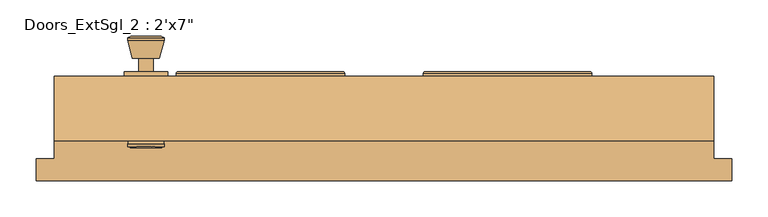
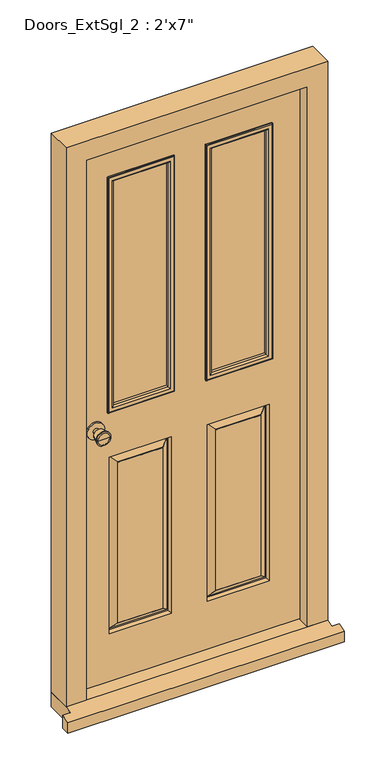
"""IFC4 building model written with IfcOpenShell, lengths in millimetres: door geometry."""

from ifc_helpers import new_model, si_unit, point, frame, frame_2d, origin, place, context, project, spatial, polyline, circle_curve, ellipse_curve, trimmed, segment, composite_curve, outline, extrude, faceted_brep, source, transform, mapped, element, save
from ifc_brep_helpers import plane_surface, cylinder_surface, revolved_surface, advanced_brep


def door_51b0c682(model_context):
    return source(origin(), model_context, "Body", "SolidModel", [
        advanced_brep(
        [(-328.5, 18.4, 1000.0), (-338.5, 18.4, 1000.0), (-318.5, 18.4, 1000.0), (-308.0241324, 67.4, 1000.0), (-348.9758676, 67.4, 1000.0), (-328.5, 67.4, 1000.0), (-303.5, 65.5721319, 1000.0), (-353.5, 65.5721319, 1000.0), (-303.5, 62.1084537, 1000.0), (-353.5, 62.1084537, 1000.0), (-309.863764, 37.4, 1000.0), (-347.136236, 37.4, 1000.0), (-318.5, 37.4, 1000.0), (-338.5, 37.4, 1000.0)],
        [
            (0, 1),
            (1, 2, circle_curve(frame((-328.5, 18.4, 1000.0), z_axis=(0.0, -1.0, 0.0), x_axis=(-1.0, 0.0, 0.0)), 10.0)),
            (2, 0),
            (2, 1, circle_curve(frame((-328.5, 18.4, 1000.0), z_axis=(0.0, -1.0, 0.0), x_axis=(-1.0, 0.0, 0.0)), 10.0)),
            (3, 4, circle_curve(frame((-328.5, 67.4, 1000.0), z_axis=(0.0, 1.0, 0.0), x_axis=(-1.0, 0.0, 0.0)), 20.4758676)),
            (4, 5),
            (5, 3),
            (4, 3, circle_curve(frame((-328.5, 67.4, 1000.0), z_axis=(0.0, 1.0, 0.0), x_axis=(-1.0, 0.0, 0.0)), 20.4758676)),
            (6, 7, circle_curve(frame((-328.5, 65.5721319, 1000.0), z_axis=(0.0, 1.0, 0.0), x_axis=(-1.0, 0.0, 0.0)), 25.0)),
            (7, 4),
            (3, 6),
            (7, 6, circle_curve(frame((-328.5, 65.5721319, 1000.0), z_axis=(0.0, 1.0, 0.0), x_axis=(-1.0, 0.0, 0.0)), 25.0)),
            (8, 9, circle_curve(frame((-328.5, 62.1084537, 1000.0), z_axis=(0.0, 1.0, 0.0), x_axis=(-1.0, 0.0, 0.0)), 25.0)),
            (9, 7),
            (6, 8),
            (9, 8, circle_curve(frame((-328.5, 62.1084537, 1000.0), z_axis=(0.0, 1.0, 0.0), x_axis=(-1.0, 0.0, 0.0)), 25.0)),
            (10, 11, circle_curve(frame((-328.5, 37.4, 1000.0), z_axis=(0.0, 1.0, 0.0), x_axis=(-1.0, 0.0, 0.0)), 18.636236)),
            (11, 9),
            (8, 10),
            (11, 10, circle_curve(frame((-328.5, 37.4, 1000.0), z_axis=(0.0, 1.0, 0.0), x_axis=(-1.0, 0.0, 0.0)), 18.636236)),
            (12, 13, circle_curve(frame((-328.5, 37.4, 1000.0), z_axis=(0.0, 1.0, 0.0), x_axis=(-1.0, 0.0, 0.0)), 10.0)),
            (13, 11),
            (10, 12),
            (13, 12, circle_curve(frame((-328.5, 37.4, 1000.0), z_axis=(0.0, 1.0, 0.0), x_axis=(-1.0, 0.0, 0.0)), 10.0)),
            (1, 13),
            (12, 2),
        ],
        [
            plane_surface(frame((-328.5, 18.4, 1000.0), z_axis=(0.0, -1.0, 0.0), x_axis=(-1.0, 0.0, 0.0))),
            plane_surface(frame((-328.5, 67.4, 1000.0), z_axis=(0.0, 1.0, 0.0), x_axis=(-1.0, 0.0, 0.0))),
            revolved_surface(polyline([(-348.9758676, 67.4, 1000.0), (-353.5, 65.5721319, 1000.0)]), (-328.5, 18.4, 1000.0), (0.0, -1.0, 0.0)),
            cylinder_surface(frame((-328.5, 18.4, 1000.0), z_axis=(0.0, -1.0, 0.0), x_axis=(-1.0, 0.0, 0.0)), 25.0),
            revolved_surface(polyline([(-353.5, 62.1084537, 1000.0), (-347.136236, 37.4, 1000.0)]), (-328.5, 18.4, 1000.0), (0.0, -1.0, 0.0)),
            plane_surface(frame((-328.5, 37.4, 1000.0), z_axis=(0.0, -1.0, 0.0), x_axis=(-1.0, 0.0, 0.0))),
            cylinder_surface(frame((-328.5, 18.4, 1000.0), z_axis=(0.0, -1.0, 0.0), x_axis=(-1.0, 0.0, 0.0)), 10.0),
        ],
        [
            (0, [[1, 2, 3]]),
            (0, [[-3, 4, -1]]),
            (1, [[5, 6, 7]]),
            (1, [[8, -7, -6]]),
            (2, [[9, 10, -5, 11]]),
            (2, [[12, -11, -8, -10]]),
            (3, [[13, 14, -9, 15]]),
            (3, [[16, -15, -12, -14]]),
            (4, [[17, 18, -13, 19]]),
            (4, [[20, -19, -16, -18]]),
            (5, [[21, 22, -17, 23]]),
            (5, [[24, -23, -20, -22]]),
            (6, [[-2, 25, -21, 26]]),
            (6, [[-4, -26, -24, -25]]),
        ],
    ),
        extrude(outline(composite_curve([segment(trimmed(circle_curve(frame_2d((1000.0, -328.5)), 30.0), [point((1000.0, -358.5))], [point((1000.0, -298.5))], False, "CARTESIAN"), True, "CONTINUOUS"), segment(trimmed(circle_curve(frame_2d((1000.0, -328.5)), 30.0), [point((1000.0, -298.5))], [point((1000.0, -358.5))], False, "CARTESIAN"), True, "CONTINUOUS")], self_intersect=False)), frame((0.0, 12.4, 0.0), z_axis=(0.0, 1.0, 0.0), x_axis=(0.0, 0.0, 1.0)), (0.0, 0.0, 1.0), 6.0),
        advanced_brep(
        [(-328.5, -37.6, 1000.0), (-318.5, -37.6, 1000.0), (-338.5, -37.6, 1000.0), (-308.0241324, -86.6, 1000.0), (-328.5, -86.6, 1000.0), (-348.9758676, -86.6, 1000.0), (-303.5, -84.7721319, 1000.0), (-353.5, -84.7721319, 1000.0), (-303.5, -81.3084537, 1000.0), (-353.5, -81.3084537, 1000.0), (-309.863764, -56.6, 1000.0), (-347.136236, -56.6, 1000.0), (-318.5, -56.6, 1000.0), (-338.5, -56.6, 1000.0)],
        [
            (0, 1),
            (1, 2, circle_curve(frame((-328.5, -37.6, 1000.0), z_axis=(0.0, 1.0, 0.0), x_axis=(-1.0, 0.0, 0.0)), 10.0)),
            (2, 0),
            (2, 1, circle_curve(frame((-328.5, -37.6, 1000.0), z_axis=(0.0, 1.0, 0.0), x_axis=(-1.0, 0.0, 0.0)), 10.0)),
            (3, 4),
            (4, 5),
            (5, 3, circle_curve(frame((-328.5, -86.6, 1000.0), z_axis=(0.0, -1.0, 0.0), x_axis=(-1.0, 0.0, 0.0)), 20.4758676)),
            (3, 5, circle_curve(frame((-328.5, -86.6, 1000.0), z_axis=(0.0, -1.0, 0.0), x_axis=(-1.0, 0.0, 0.0)), 20.4758676)),
            (6, 3),
            (5, 7),
            (7, 6, circle_curve(frame((-328.5, -84.7721319, 1000.0), z_axis=(0.0, -1.0, 0.0), x_axis=(-1.0, 0.0, 0.0)), 25.0)),
            (6, 7, circle_curve(frame((-328.5, -84.7721319, 1000.0), z_axis=(0.0, -1.0, 0.0), x_axis=(-1.0, 0.0, 0.0)), 25.0)),
            (8, 6),
            (7, 9),
            (9, 8, circle_curve(frame((-328.5, -81.3084537, 1000.0), z_axis=(0.0, -1.0, 0.0), x_axis=(-1.0, 0.0, 0.0)), 25.0)),
            (8, 9, circle_curve(frame((-328.5, -81.3084537, 1000.0), z_axis=(0.0, -1.0, 0.0), x_axis=(-1.0, 0.0, 0.0)), 25.0)),
            (10, 8),
            (9, 11),
            (11, 10, circle_curve(frame((-328.5, -56.6, 1000.0), z_axis=(0.0, -1.0, 0.0), x_axis=(-1.0, 0.0, 0.0)), 18.636236)),
            (10, 11, circle_curve(frame((-328.5, -56.6, 1000.0), z_axis=(0.0, -1.0, 0.0), x_axis=(-1.0, 0.0, 0.0)), 18.636236)),
            (12, 10),
            (11, 13),
            (13, 12, circle_curve(frame((-328.5, -56.6, 1000.0), z_axis=(0.0, -1.0, 0.0), x_axis=(-1.0, 0.0, 0.0)), 10.0)),
            (12, 13, circle_curve(frame((-328.5, -56.6, 1000.0), z_axis=(0.0, -1.0, 0.0), x_axis=(-1.0, 0.0, 0.0)), 10.0)),
            (1, 12),
            (13, 2),
        ],
        [
            plane_surface(frame((-328.5, -37.6, 1000.0), z_axis=(0.0, 1.0, 0.0), x_axis=(-1.0, 0.0, 0.0))),
            plane_surface(frame((-328.5, -86.6, 1000.0), z_axis=(0.0, -1.0, 0.0), x_axis=(-1.0, 0.0, 0.0))),
            revolved_surface(polyline([(-348.9758676, -86.6, 1000.0), (-353.5, -84.7721319, 1000.0)]), (-328.5, -37.6, 1000.0), (0.0, 1.0, 0.0)),
            cylinder_surface(frame((-328.5, -37.6, 1000.0), z_axis=(0.0, 1.0, 0.0), x_axis=(-1.0, 0.0, 0.0)), 25.0),
            revolved_surface(polyline([(-353.5, -81.3084537, 1000.0), (-347.136236, -56.6, 1000.0)]), (-328.5, -37.6, 1000.0), (0.0, 1.0, 0.0)),
            plane_surface(frame((-328.5, -56.6, 1000.0), z_axis=(0.0, 1.0, 0.0), x_axis=(-1.0, 0.0, 0.0))),
            cylinder_surface(frame((-328.5, -37.6, 1000.0), z_axis=(0.0, 1.0, 0.0), x_axis=(-1.0, 0.0, 0.0)), 10.0),
        ],
        [
            (0, [[1, 2, 3]]),
            (0, [[-3, 4, -1]]),
            (1, [[5, 6, 7]]),
            (1, [[-6, -5, 8]]),
            (2, [[9, -7, 10, 11]]),
            (2, [[-10, -8, -9, 12]]),
            (3, [[13, -11, 14, 15]]),
            (3, [[-14, -12, -13, 16]]),
            (4, [[17, -15, 18, 19]]),
            (4, [[-18, -16, -17, 20]]),
            (5, [[21, -19, 22, 23]]),
            (5, [[-22, -20, -21, 24]]),
            (6, [[25, -23, 26, -2]]),
            (6, [[-26, -24, -25, -4]]),
        ],
    ),
        extrude(outline(composite_curve([segment(trimmed(circle_curve(frame_2d((1000.0, -328.5)), 30.0), [point((1000.0, -358.5))], [point((1000.0, -298.5))], False, "CARTESIAN"), True, "CONTINUOUS"), segment(trimmed(circle_curve(frame_2d((1000.0, -328.5)), 30.0), [point((1000.0, -298.5))], [point((1000.0, -358.5))], False, "CARTESIAN"), True, "CONTINUOUS")], self_intersect=False)), frame((0.0, -37.6, 0.0), z_axis=(0.0, 1.0, 0.0), x_axis=(0.0, 0.0, 1.0)), (0.0, 0.0, 1.0), 6.0),
        faceted_brep([(384.5, -76.6, 54.5), (384.5, -34.6, 54.5), (406.5, -34.6, 54.5), (406.5, 12.4, 54.5), (455.0, 12.4, 54.5), (455.0, -76.6, 54.5), (455.0, -76.6, 2110.0), (-455.0, -76.6, 2110.0), (-455.0, -76.6, 54.5), (-384.5, -76.6, 54.5), (-384.5, -76.6, 2039.5), (384.5, -76.6, 2039.5), (455.0, 12.4, 2110.0), (406.5, 12.4, 2061.5), (-406.5, 12.4, 2061.5), (-406.5, 12.4, 54.5), (-455.0, 12.4, 54.5), (-455.0, 12.4, 2110.0), (406.5, -34.6, 2061.5), (384.5, -34.6, 2039.5), (-384.5, -34.6, 2039.5), (-384.5, -34.6, 54.5), (-406.5, -34.6, 54.5), (-406.5, -34.6, 2061.5)], [[[0, 1, 2, 3, 4, 5]], [[5, 6, 7, 8, 9, 10, 11, 0]], [[4, 12, 6, 5]], [[3, 13, 14, 15, 16, 17, 12, 4]], [[2, 18, 13, 3]], [[1, 19, 20, 21, 22, 23, 18, 2]], [[0, 11, 19, 1]], [[9, 21, 20, 10]], [[8, 16, 15, 22, 21, 9]], [[7, 17, 16, 8]], [[14, 23, 22, 15]], [[6, 12, 17, 7]], [[13, 18, 23, 14]], [[10, 20, 19, 11]]]),
        faceted_brep([(403.5, 12.4, 58.5), (-404.4250294, 12.4, 58.5), (-404.4250294, 12.4, 2058.5), (403.5, 12.4, 2058.5), (62.5, 12.4, 1058.5), (278.5, 12.4, 1058.5), (278.5, 12.4, 1908.5), (62.5, 12.4, 1908.5), (-278.5, 12.4, 1058.5), (-62.5, 12.4, 1058.5), (-62.5, 12.4, 1908.5), (-278.5, 12.4, 1908.5), (-62.5, 12.4, 883.5), (-278.5, 12.4, 883.5), (-278.5, 12.4, 233.5), (-62.5, 12.4, 233.5), (278.5, 12.4, 883.5), (62.5, 12.4, 883.5), (62.5, 12.4, 233.5), (278.5, 12.4, 233.5), (-92.5, 12.4, 263.5), (-248.5, 12.4, 263.5), (-248.5, 12.4, 853.5), (-92.5, 12.4, 853.5), (248.5, 12.4, 263.5), (92.5, 12.4, 263.5), (92.5, 12.4, 853.5), (248.5, 12.4, 853.5), (403.5, -31.6, 58.5), (403.5, -31.6, 2058.5), (-404.4250294, -31.6, 2058.5), (-404.4250294, -31.6, 58.5), (62.5, -31.6, 1058.5), (62.5, -31.6, 1908.5), (278.5, -31.6, 1908.5), (278.5, -31.6, 1058.5), (-278.5, -31.6, 1058.5), (-278.5, -31.6, 1908.5), (-62.5, -31.6, 1908.5), (-62.5, -31.6, 1058.5), (62.5, -31.6, 883.5), (278.5, -31.6, 883.5), (278.5, -31.6, 233.5), (62.5, -31.6, 233.5), (-278.5, -31.6, 883.5), (-62.5, -31.6, 883.5), (-62.5, -31.6, 233.5), (-278.5, -31.6, 233.5), (92.5, -31.6, 263.5), (248.5, -31.6, 263.5), (248.5, -31.6, 853.5), (92.5, -31.6, 853.5), (-248.5, -31.6, 263.5), (-92.5, -31.6, 263.5), (-92.5, -31.6, 853.5), (-248.5, -31.6, 853.5), (65.5, -16.6, 880.5), (65.5, -16.6, 236.5), (90.5, -30.6, 855.5), (70.5, -16.6, 875.5), (70.5, -16.6, 241.5), (90.5, -30.6, 261.5), (92.5, -30.6, 853.5), (92.5, -30.6, 263.5), (275.5, -16.6, 236.5), (270.5, -16.6, 241.5), (250.5, -30.6, 261.5), (248.5, -30.6, 263.5), (275.5, -16.6, 880.5), (270.5, -16.6, 875.5), (250.5, -30.6, 855.5), (248.5, -30.6, 853.5), (-275.5, -16.6, 880.5), (-275.5, -16.6, 236.5), (-250.5, -30.6, 855.5), (-270.5, -16.6, 875.5), (-270.5, -16.6, 241.5), (-250.5, -30.6, 261.5), (-248.5, -30.6, 853.5), (-248.5, -30.6, 263.5), (-65.5, -16.6, 236.5), (-70.5, -16.6, 241.5), (-90.5, -30.6, 261.5), (-92.5, -30.6, 263.5), (-65.5, -16.6, 880.5), (-70.5, -16.6, 875.5), (-90.5, -30.6, 855.5), (-92.5, -30.6, 853.5), (-92.5, 11.4, 263.5), (-92.5, 11.4, 853.5), (-70.5, -2.6, 241.5), (-90.5, 11.4, 261.5), (-90.5, 11.4, 855.5), (-70.5, -2.6, 875.5), (-65.5, -2.6, 236.5), (-65.5, -2.6, 880.5), (-248.5, 11.4, 853.5), (-250.5, 11.4, 855.5), (-270.5, -2.6, 875.5), (-275.5, -2.6, 880.5), (-248.5, 11.4, 263.5), (-250.5, 11.4, 261.5), (-270.5, -2.6, 241.5), (-275.5, -2.6, 236.5), (275.5, -2.6, 880.5), (275.5, -2.6, 236.5), (250.5, 11.4, 855.5), (270.5, -2.6, 875.5), (270.5, -2.6, 241.5), (250.5, 11.4, 261.5), (248.5, 11.4, 853.5), (248.5, 11.4, 263.5), (65.5, -2.6, 236.5), (70.5, -2.6, 241.5), (90.5, 11.4, 261.5), (92.5, 11.4, 263.5), (65.5, -2.6, 880.5), (70.5, -2.6, 875.5), (90.5, 11.4, 855.5), (92.5, 11.4, 853.5)], [[[0, 1, 2, 3], [4, 5, 6, 7], [8, 9, 10, 11], [12, 13, 14, 15], [16, 17, 18, 19]], [[20, 21, 22, 23]], [[24, 25, 26, 27]], [[28, 29, 30, 31], [32, 33, 34, 35], [36, 37, 38, 39], [40, 41, 42, 43], [44, 45, 46, 47]], [[48, 49, 50, 51]], [[52, 53, 54, 55]], [[3, 29, 28, 0]], [[2, 30, 29, 3]], [[1, 31, 30, 2]], [[0, 28, 31, 1]], [[7, 33, 32, 4]], [[6, 34, 33, 7]], [[5, 35, 34, 6]], [[4, 32, 35, 5]], [[11, 37, 36, 8]], [[10, 38, 37, 11]], [[9, 39, 38, 10]], [[8, 36, 39, 9]], [[56, 40, 43, 57]], [[58, 59, 60, 61]], [[48, 51, 62, 63]], [[43, 42, 64, 57]], [[60, 65, 66, 61]], [[63, 67, 49, 48]], [[42, 41, 68, 64]], [[65, 69, 70, 66]], [[67, 71, 50, 49]], [[56, 68, 41, 40]], [[57, 64, 68, 56], [59, 69, 65, 60]], [[58, 70, 69, 59]], [[61, 66, 70, 58], [62, 71, 67, 63]], [[51, 50, 71, 62]], [[72, 44, 47, 73]], [[74, 75, 76, 77]], [[52, 55, 78, 79]], [[47, 46, 80, 73]], [[76, 81, 82, 77]], [[79, 83, 53, 52]], [[46, 45, 84, 80]], [[81, 85, 86, 82]], [[83, 87, 54, 53]], [[72, 84, 45, 44]], [[73, 80, 84, 72], [75, 85, 81, 76]], [[74, 86, 85, 75]], [[77, 82, 86, 74], [78, 87, 83, 79]], [[55, 54, 87, 78]], [[88, 20, 23, 89]], [[90, 91, 92, 93]], [[12, 15, 94, 95]], [[23, 22, 96, 89]], [[92, 97, 98, 93]], [[95, 99, 13, 12]], [[22, 21, 100, 96]], [[97, 101, 102, 98]], [[99, 103, 14, 13]], [[88, 100, 21, 20]], [[91, 101, 97, 92], [89, 96, 100, 88]], [[90, 102, 101, 91]], [[94, 103, 99, 95], [93, 98, 102, 90]], [[15, 14, 103, 94]], [[104, 16, 19, 105]], [[106, 107, 108, 109]], [[24, 27, 110, 111]], [[19, 18, 112, 105]], [[108, 113, 114, 109]], [[111, 115, 25, 24]], [[18, 17, 116, 112]], [[113, 117, 118, 114]], [[115, 119, 26, 25]], [[104, 116, 17, 16]], [[105, 112, 116, 104], [107, 117, 113, 108]], [[106, 118, 117, 107]], [[109, 114, 118, 106], [110, 119, 115, 111]], [[27, 26, 119, 110]]]),
        faceted_brep([(480.0, -131.6, 0.0), (480.0, -101.6, 0.0), (480.0, -101.6, 47.2703282), (480.0, -131.6, 38.5947221), (-480.0, -131.6, 38.5947221), (-480.0, -101.6, 47.2703282), (-480.0, -101.6, 0.0), (-480.0, -131.6, 0.0), (-455.0, -101.6, 0.0), (-455.0, 12.4, 0.0), (455.0, 12.4, 0.0), (455.0, -101.6, 0.0), (455.0, -101.6, 47.2703282), (455.0, -76.6, 54.5), (-455.0, -76.6, 54.5), (-455.0, -101.6, 47.2703282), (455.0, 12.4, 54.5), (-455.0, 12.4, 54.5)], [[[0, 1, 2, 3]], [[4, 5, 6, 7]], [[7, 6, 8, 9, 10, 11, 1, 0]], [[3, 4, 7, 0]], [[3, 2, 12, 13, 14, 15, 5, 4]], [[14, 13, 16, 17]], [[17, 16, 10, 9]], [[15, 14, 17, 9, 8]], [[8, 6, 5, 15]], [[11, 10, 16, 13, 12]], [[12, 2, 1, 11]]]),
        extrude(outline(polyline([(278.5, 2.4), (278.5, -21.6), (62.5, -21.6), (62.5, 2.4), (278.5, 2.4)])), frame((0.0, 0.0, 1058.5), z_axis=(0.0, 0.0, 1.0), x_axis=(1.0, 0.0, 0.0)), (0.0, 0.0, 1.0), 850.0),
        extrude(outline(polyline([(-62.5, 2.4), (-62.5, -21.6), (-278.5, -21.6), (-278.5, 2.4), (-62.5, 2.4)])), frame((0.0, 0.0, 1058.5), z_axis=(0.0, 0.0, 1.0), x_axis=(1.0, 0.0, 0.0)), (0.0, 0.0, 1.0), 850.0),
        advanced_brep(
        [(286.5, -35.6, 1916.5), (286.5, -35.6, 1050.5), (286.5, -31.6, 1050.5), (286.5, -31.6, 1916.5), (284.5, -37.6, 1914.5), (284.5, -37.6, 1052.5), (266.5, -32.6, 1896.5), (266.5, -32.6, 1070.5), (271.5, -37.6, 1065.5), (271.5, -37.6, 1901.5), (266.5, -21.6, 1896.5), (266.5, -21.6, 1070.5), (278.5, -31.6, 1908.5), (278.5, -31.6, 1058.5), (278.5, -21.6, 1058.5), (278.5, -21.6, 1908.5), (54.5, -35.6, 1050.5), (54.5, -31.6, 1050.5), (56.5, -37.6, 1052.5), (74.5, -32.6, 1070.5), (69.5, -37.6, 1065.5), (74.5, -21.6, 1070.5), (62.5, -31.6, 1058.5), (62.5, -21.6, 1058.5), (54.5, -35.6, 1916.5), (54.5, -31.6, 1916.5), (56.5, -37.6, 1914.5), (74.5, -32.6, 1896.5), (69.5, -37.6, 1901.5), (74.5, -21.6, 1896.5), (62.5, -31.6, 1908.5), (62.5, -21.6, 1908.5)],
        [
            (0, 1),
            (1, 2),
            (2, 3),
            (3, 0),
            (4, 5),
            (5, 1, ellipse_curve(frame((284.5, -35.6, 1052.5), z_axis=(0.7071067811865475, 0.0, 0.7071067811865475), x_axis=(-0.7071067811865474, 0.0, 0.7071067811865476)), 2.8284271, 2.0)),
            (0, 4, ellipse_curve(frame((284.5, -35.6, 1914.5), z_axis=(0.7071067811865475, 0.0, -0.7071067811865475), x_axis=(0.7071067811865474, 0.0, 0.7071067811865476)), 2.8284271, 2.0)),
            (6, 7),
            (7, 8, ellipse_curve(frame((271.5, -32.6, 1065.5), z_axis=(0.7071067811865475, 0.0, 0.7071067811865475), x_axis=(-0.7071067811865474, 0.0, 0.7071067811865476)), 7.0710678, 5.0)),
            (8, 9),
            (9, 6, ellipse_curve(frame((271.5, -32.6, 1901.5), z_axis=(0.7071067811865475, 0.0, -0.7071067811865475), x_axis=(0.7071067811865474, 0.0, 0.7071067811865476)), 7.0710678, 5.0)),
            (10, 11),
            (11, 7),
            (6, 10),
            (12, 13),
            (13, 14),
            (14, 15),
            (15, 12),
            (1, 16),
            (16, 17),
            (17, 2),
            (5, 18),
            (18, 16, ellipse_curve(frame((56.5, -35.6, 1052.5), z_axis=(0.7071067811865475, 0.0, -0.7071067811865475), x_axis=(0.7071067811865476, 0.0, 0.7071067811865474)), 2.8284271, 2.0)),
            (7, 19),
            (19, 20, ellipse_curve(frame((69.5, -32.6, 1065.5), z_axis=(0.7071067811865475, 0.0, -0.7071067811865475), x_axis=(0.7071067811865476, 0.0, 0.7071067811865474)), 7.0710678, 5.0)),
            (20, 8),
            (11, 21),
            (21, 19),
            (13, 22),
            (22, 23),
            (23, 14),
            (16, 24),
            (24, 25),
            (25, 17),
            (18, 26),
            (26, 24, ellipse_curve(frame((56.5, -35.6, 1914.5), z_axis=(-0.7071067811865475, 0.0, -0.7071067811865475), x_axis=(0.7071067811865474, 0.0, -0.7071067811865476)), 2.8284271, 2.0)),
            (19, 27),
            (27, 28, ellipse_curve(frame((69.5, -32.6, 1901.5), z_axis=(-0.7071067811865475, 0.0, -0.7071067811865475), x_axis=(0.7071067811865474, 0.0, -0.7071067811865476)), 7.0710678, 5.0)),
            (28, 20),
            (21, 29),
            (29, 27),
            (22, 30),
            (30, 31),
            (31, 23),
            (24, 0),
            (3, 25),
            (26, 4),
            (28, 9),
            (27, 6),
            (29, 10),
            (31, 15),
            (30, 12),
        ],
        [
            plane_surface(frame((286.5, -31.6, 1916.5), z_axis=(1.0, 0.0, 0.0), x_axis=(0.0, 0.0, -1.0))),
            cylinder_surface(frame((284.5, -35.6, 1908.5), z_axis=(0.0, 0.0, 1.0), x_axis=(1.0, 0.0, 0.0)), 2.0),
            cylinder_surface(frame((271.5, -32.6, 1908.5), z_axis=(0.0, 0.0, 1.0), x_axis=(1.0, 0.0, 0.0)), 5.0),
            plane_surface(frame((266.5, -32.6, 1896.5), z_axis=(-1.0, 0.0, 0.0), x_axis=(0.0, 0.0, -1.0))),
            plane_surface(frame((278.5, -21.6, 1908.5), z_axis=(1.0, 0.0, 0.0), x_axis=(0.0, 0.0, -1.0))),
            plane_surface(frame((286.5, -31.6, 1050.5), z_axis=(0.0, 0.0, -1.0), x_axis=(-1.0, 0.0, 0.0))),
            cylinder_surface(frame((278.5, -35.6, 1052.5), z_axis=(1.0, 0.0, 0.0), x_axis=(0.0, 0.0, -1.0)), 2.0),
            cylinder_surface(frame((278.5, -32.6, 1065.5), z_axis=(1.0, 0.0, 0.0), x_axis=(0.0, 0.0, -1.0)), 5.0),
            plane_surface(frame((266.5, -32.6, 1070.5), z_axis=(0.0, 0.0, 1.0), x_axis=(-1.0, 0.0, 0.0))),
            plane_surface(frame((278.5, -21.6, 1058.5), z_axis=(0.0, 0.0, -1.0), x_axis=(-1.0, 0.0, 0.0))),
            plane_surface(frame((54.5, -31.6, 1050.5), z_axis=(-1.0, 0.0, 0.0), x_axis=(0.0, 0.0, 1.0))),
            cylinder_surface(frame((56.5, -35.6, 1058.5), z_axis=(0.0, 0.0, -1.0), x_axis=(-1.0, 0.0, 0.0)), 2.0),
            cylinder_surface(frame((69.5, -32.6, 1058.5), z_axis=(0.0, 0.0, -1.0), x_axis=(-1.0, 0.0, 0.0)), 5.0),
            plane_surface(frame((74.5, -32.6, 1070.5), z_axis=(1.0, 0.0, 0.0), x_axis=(0.0, 0.0, 1.0))),
            plane_surface(frame((62.5, -21.6, 1058.5), z_axis=(-1.0, 0.0, 0.0), x_axis=(0.0, 0.0, 1.0))),
            plane_surface(frame((54.5, -31.6, 1916.5), z_axis=(0.0, 0.0, 1.0), x_axis=(1.0, 0.0, 0.0))),
            cylinder_surface(frame((62.5, -35.6, 1914.5), z_axis=(-1.0, 0.0, 0.0), x_axis=(0.0, 0.0, 1.0)), 2.0),
            plane_surface(frame((56.5, -37.6, 1914.5), z_axis=(0.0, -1.0, 0.0), x_axis=(1.0, 0.0, 0.0))),
            cylinder_surface(frame((62.5, -32.6, 1901.5), z_axis=(-1.0, 0.0, 0.0), x_axis=(0.0, 0.0, 1.0)), 5.0),
            plane_surface(frame((74.5, -32.6, 1896.5), z_axis=(0.0, 0.0, -1.0), x_axis=(1.0, 0.0, 0.0))),
            plane_surface(frame((74.5, -21.6, 1896.5), z_axis=(0.0, 1.0, 0.0), x_axis=(1.0, 0.0, 0.0))),
            plane_surface(frame((62.5, -21.6, 1908.5), z_axis=(0.0, 0.0, 1.0), x_axis=(1.0, 0.0, 0.0))),
            plane_surface(frame((62.5, -31.6, 1908.5), z_axis=(0.0, 1.0, 0.0), x_axis=(1.0, 0.0, 0.0))),
        ],
        [
            (0, [[1, 2, 3, 4]]),
            (1, [[5, 6, -1, 7]]),
            (2, [[8, 9, 10, 11]]),
            (3, [[12, 13, -8, 14]]),
            (4, [[15, 16, 17, 18]]),
            (5, [[19, 20, 21, -2]]),
            (6, [[22, 23, -19, -6]]),
            (7, [[24, 25, 26, -9]]),
            (8, [[27, 28, -24, -13]]),
            (9, [[29, 30, 31, -16]]),
            (10, [[32, 33, 34, -20]]),
            (11, [[35, 36, -32, -23]]),
            (12, [[37, 38, 39, -25]]),
            (13, [[40, 41, -37, -28]]),
            (14, [[42, 43, 44, -30]]),
            (15, [[45, -4, 46, -33]]),
            (16, [[47, -7, -45, -36]]),
            (17, [[-5, -47, -35, -22], [-10, -26, -39, 48]]),
            (18, [[49, -11, -48, -38]]),
            (19, [[50, -14, -49, -41]]),
            (20, [[-17, -31, -44, 51], [-12, -50, -40, -27]]),
            (21, [[52, -18, -51, -43]]),
            (22, [[-3, -21, -34, -46], [-15, -52, -42, -29]]),
        ],
    ),
        advanced_brep(
        [(-54.5, -35.6, 1050.5), (-286.5, -35.6, 1050.5), (-286.5, -31.6, 1050.5), (-54.5, -31.6, 1050.5), (-56.5, -37.6, 1052.5), (-284.5, -37.6, 1052.5), (-74.5, -32.6, 1070.5), (-266.5, -32.6, 1070.5), (-271.5, -37.6, 1065.5), (-69.5, -37.6, 1065.5), (-74.5, -21.6, 1070.5), (-266.5, -21.6, 1070.5), (-62.5, -31.6, 1058.5), (-278.5, -31.6, 1058.5), (-278.5, -21.6, 1058.5), (-62.5, -21.6, 1058.5), (-286.5, -35.6, 1916.5), (-286.5, -31.6, 1916.5), (-284.5, -37.6, 1914.5), (-266.5, -32.6, 1896.5), (-271.5, -37.6, 1901.5), (-266.5, -21.6, 1896.5), (-278.5, -31.6, 1908.5), (-278.5, -21.6, 1908.5), (-54.5, -35.6, 1916.5), (-54.5, -31.6, 1916.5), (-56.5, -37.6, 1914.5), (-74.5, -32.6, 1896.5), (-69.5, -37.6, 1901.5), (-74.5, -21.6, 1896.5), (-62.5, -31.6, 1908.5), (-62.5, -21.6, 1908.5)],
        [
            (0, 1),
            (1, 2),
            (2, 3),
            (3, 0),
            (4, 5),
            (5, 1, ellipse_curve(frame((-284.5, -35.6, 1052.5), z_axis=(0.7071067811865475, 0.0, -0.7071067811865475), x_axis=(0.7071067811865476, 0.0, 0.7071067811865474)), 2.8284271, 2.0)),
            (0, 4, ellipse_curve(frame((-56.5, -35.6, 1052.5), z_axis=(-0.7071067811865475, 0.0, -0.7071067811865475), x_axis=(0.7071067811865476, 0.0, -0.7071067811865474)), 2.8284271, 2.0)),
            (6, 7),
            (7, 8, ellipse_curve(frame((-271.5, -32.6, 1065.5), z_axis=(0.7071067811865475, 0.0, -0.7071067811865475), x_axis=(0.7071067811865476, 0.0, 0.7071067811865474)), 7.0710678, 5.0)),
            (8, 9),
            (9, 6, ellipse_curve(frame((-69.5, -32.6, 1065.5), z_axis=(-0.7071067811865475, 0.0, -0.7071067811865475), x_axis=(0.7071067811865476, 0.0, -0.7071067811865474)), 7.0710678, 5.0)),
            (10, 11),
            (11, 7),
            (6, 10),
            (12, 13),
            (13, 14),
            (14, 15),
            (15, 12),
            (1, 16),
            (16, 17),
            (17, 2),
            (5, 18),
            (18, 16, ellipse_curve(frame((-284.5, -35.6, 1914.5), z_axis=(-0.7071067811865475, 0.0, -0.7071067811865475), x_axis=(0.7071067811865474, 0.0, -0.7071067811865476)), 2.8284271, 2.0)),
            (7, 19),
            (19, 20, ellipse_curve(frame((-271.5, -32.6, 1901.5), z_axis=(-0.7071067811865475, 0.0, -0.7071067811865475), x_axis=(0.7071067811865474, 0.0, -0.7071067811865476)), 7.0710678, 5.0)),
            (20, 8),
            (11, 21),
            (21, 19),
            (13, 22),
            (22, 23),
            (23, 14),
            (16, 24),
            (24, 25),
            (25, 17),
            (18, 26),
            (26, 24, ellipse_curve(frame((-56.5, -35.6, 1914.5), z_axis=(-0.7071067811865475, 0.0, 0.7071067811865475), x_axis=(-0.7071067811865476, 0.0, -0.7071067811865474)), 2.8284271, 2.0)),
            (19, 27),
            (27, 28, ellipse_curve(frame((-69.5, -32.6, 1901.5), z_axis=(-0.7071067811865475, 0.0, 0.7071067811865475), x_axis=(-0.7071067811865476, 0.0, -0.7071067811865474)), 7.0710678, 5.0)),
            (28, 20),
            (21, 29),
            (29, 27),
            (22, 30),
            (30, 31),
            (31, 23),
            (24, 0),
            (3, 25),
            (26, 4),
            (28, 9),
            (27, 6),
            (29, 10),
            (31, 15),
            (30, 12),
        ],
        [
            plane_surface(frame((-54.5, -31.6, 1050.5), z_axis=(0.0, 0.0, -1.0), x_axis=(-1.0, 0.0, 0.0))),
            cylinder_surface(frame((-62.5, -35.6, 1052.5), z_axis=(1.0, 0.0, 0.0), x_axis=(0.0, 0.0, -1.0)), 2.0),
            cylinder_surface(frame((-62.5, -32.6, 1065.5), z_axis=(1.0, 0.0, 0.0), x_axis=(0.0, 0.0, -1.0)), 5.0),
            plane_surface(frame((-74.5, -32.6, 1070.5), z_axis=(0.0, 0.0, 1.0), x_axis=(-1.0, 0.0, 0.0))),
            plane_surface(frame((-62.5, -21.6, 1058.5), z_axis=(0.0, 0.0, -1.0), x_axis=(-1.0, 0.0, 0.0))),
            plane_surface(frame((-286.5, -31.6, 1050.5), z_axis=(-1.0, 0.0, 0.0), x_axis=(0.0, 0.0, 1.0))),
            cylinder_surface(frame((-284.5, -35.6, 1058.5), z_axis=(0.0, 0.0, -1.0), x_axis=(-1.0, 0.0, 0.0)), 2.0),
            cylinder_surface(frame((-271.5, -32.6, 1058.5), z_axis=(0.0, 0.0, -1.0), x_axis=(-1.0, 0.0, 0.0)), 5.0),
            plane_surface(frame((-266.5, -32.6, 1070.5), z_axis=(1.0, 0.0, 0.0), x_axis=(0.0, 0.0, 1.0))),
            plane_surface(frame((-278.5, -21.6, 1058.5), z_axis=(-1.0, 0.0, 0.0), x_axis=(0.0, 0.0, 1.0))),
            plane_surface(frame((-286.5, -31.6, 1916.5), z_axis=(0.0, 0.0, 1.0), x_axis=(1.0, 0.0, 0.0))),
            cylinder_surface(frame((-278.5, -35.6, 1914.5), z_axis=(-1.0, 0.0, 0.0), x_axis=(0.0, 0.0, 1.0)), 2.0),
            cylinder_surface(frame((-278.5, -32.6, 1901.5), z_axis=(-1.0, 0.0, 0.0), x_axis=(0.0, 0.0, 1.0)), 5.0),
            plane_surface(frame((-266.5, -32.6, 1896.5), z_axis=(0.0, 0.0, -1.0), x_axis=(1.0, 0.0, 0.0))),
            plane_surface(frame((-278.5, -21.6, 1908.5), z_axis=(0.0, 0.0, 1.0), x_axis=(1.0, 0.0, 0.0))),
            plane_surface(frame((-54.5, -31.6, 1916.5), z_axis=(1.0, 0.0, 0.0), x_axis=(0.0, 0.0, -1.0))),
            cylinder_surface(frame((-56.5, -35.6, 1908.5), z_axis=(0.0, 0.0, 1.0), x_axis=(1.0, 0.0, 0.0)), 2.0),
            plane_surface(frame((-56.5, -37.6, 1914.5), z_axis=(0.0, -1.0, 0.0), x_axis=(0.0, 0.0, -1.0))),
            cylinder_surface(frame((-69.5, -32.6, 1908.5), z_axis=(0.0, 0.0, 1.0), x_axis=(1.0, 0.0, 0.0)), 5.0),
            plane_surface(frame((-74.5, -32.6, 1896.5), z_axis=(-1.0, 0.0, 0.0), x_axis=(0.0, 0.0, -1.0))),
            plane_surface(frame((-74.5, -21.6, 1896.5), z_axis=(0.0, 1.0, 0.0), x_axis=(0.0, 0.0, -1.0))),
            plane_surface(frame((-62.5, -21.6, 1908.5), z_axis=(1.0, 0.0, 0.0), x_axis=(0.0, 0.0, -1.0))),
            plane_surface(frame((-62.5, -31.6, 1908.5), z_axis=(0.0, 1.0, 0.0), x_axis=(0.0, 0.0, -1.0))),
        ],
        [
            (0, [[1, 2, 3, 4]]),
            (1, [[5, 6, -1, 7]]),
            (2, [[8, 9, 10, 11]]),
            (3, [[12, 13, -8, 14]]),
            (4, [[15, 16, 17, 18]]),
            (5, [[19, 20, 21, -2]]),
            (6, [[22, 23, -19, -6]]),
            (7, [[24, 25, 26, -9]]),
            (8, [[27, 28, -24, -13]]),
            (9, [[29, 30, 31, -16]]),
            (10, [[32, 33, 34, -20]]),
            (11, [[35, 36, -32, -23]]),
            (12, [[37, 38, 39, -25]]),
            (13, [[40, 41, -37, -28]]),
            (14, [[42, 43, 44, -30]]),
            (15, [[45, -4, 46, -33]]),
            (16, [[47, -7, -45, -36]]),
            (17, [[-5, -47, -35, -22], [-10, -26, -39, 48]]),
            (18, [[49, -11, -48, -38]]),
            (19, [[50, -14, -49, -41]]),
            (20, [[-17, -31, -44, 51], [-12, -50, -40, -27]]),
            (21, [[52, -18, -51, -43]]),
            (22, [[-3, -21, -34, -46], [-15, -52, -42, -29]]),
        ],
    ),
        advanced_brep(
        [(-278.5, 2.4, 1908.5), (-62.5, 2.4, 1908.5), (-62.5, 12.4, 1908.5), (-278.5, 12.4, 1908.5), (-266.5, 13.4, 1896.5), (-74.5, 13.4, 1896.5), (-74.5, 2.4, 1896.5), (-266.5, 2.4, 1896.5), (-271.5, 18.4, 1901.5), (-69.5, 18.4, 1901.5), (-286.5, 16.4, 1916.5), (-54.5, 16.4, 1916.5), (-56.5, 18.4, 1914.5), (-284.5, 18.4, 1914.5), (-286.5, 12.4, 1916.5), (-54.5, 12.4, 1916.5), (-62.5, 2.4, 1058.5), (-62.5, 12.4, 1058.5), (-74.5, 13.4, 1070.5), (-74.5, 2.4, 1070.5), (-69.5, 18.4, 1065.5), (-54.5, 16.4, 1050.5), (-56.5, 18.4, 1052.5), (-54.5, 12.4, 1050.5), (-278.5, 2.4, 1058.5), (-278.5, 12.4, 1058.5), (-266.5, 13.4, 1070.5), (-266.5, 2.4, 1070.5), (-271.5, 18.4, 1065.5), (-286.5, 16.4, 1050.5), (-284.5, 18.4, 1052.5), (-286.5, 12.4, 1050.5)],
        [
            (0, 1),
            (1, 2),
            (2, 3),
            (3, 0),
            (4, 5),
            (5, 6),
            (6, 7),
            (7, 4),
            (8, 9),
            (9, 5, ellipse_curve(frame((-69.5, 13.4, 1901.5), z_axis=(-0.7071067811865475, 0.0, 0.7071067811865475), x_axis=(-0.7071067811865476, 0.0, -0.7071067811865474)), 7.0710678, 5.0)),
            (4, 8, ellipse_curve(frame((-271.5, 13.4, 1901.5), z_axis=(0.7071067811865475, 0.0, 0.7071067811865475), x_axis=(-0.7071067811865476, 0.0, 0.7071067811865474)), 7.0710678, 5.0)),
            (10, 11),
            (11, 12, ellipse_curve(frame((-56.5, 16.4, 1914.5), z_axis=(-0.7071067811865475, 0.0, 0.7071067811865475), x_axis=(-0.7071067811865476, 0.0, -0.7071067811865474)), 2.8284271, 2.0)),
            (12, 13),
            (13, 10, ellipse_curve(frame((-284.5, 16.4, 1914.5), z_axis=(0.7071067811865475, 0.0, 0.7071067811865475), x_axis=(-0.7071067811865476, 0.0, 0.7071067811865474)), 2.8284271, 2.0)),
            (14, 15),
            (15, 11),
            (10, 14),
            (1, 16),
            (16, 17),
            (17, 2),
            (5, 18),
            (18, 19),
            (19, 6),
            (9, 20),
            (20, 18, ellipse_curve(frame((-69.5, 13.4, 1065.5), z_axis=(0.7071067811865475, 0.0, 0.7071067811865475), x_axis=(-0.7071067811865474, 0.0, 0.7071067811865476)), 7.0710678, 5.0)),
            (11, 21),
            (21, 22, ellipse_curve(frame((-56.5, 16.4, 1052.5), z_axis=(0.7071067811865475, 0.0, 0.7071067811865475), x_axis=(-0.7071067811865474, 0.0, 0.7071067811865476)), 2.8284271, 2.0)),
            (22, 12),
            (15, 23),
            (23, 21),
            (16, 24),
            (24, 25),
            (25, 17),
            (18, 26),
            (26, 27),
            (27, 19),
            (20, 28),
            (28, 26, ellipse_curve(frame((-271.5, 13.4, 1065.5), z_axis=(0.7071067811865475, 0.0, -0.7071067811865475), x_axis=(0.7071067811865476, 0.0, 0.7071067811865474)), 7.0710678, 5.0)),
            (21, 29),
            (29, 30, ellipse_curve(frame((-284.5, 16.4, 1052.5), z_axis=(0.7071067811865475, 0.0, -0.7071067811865475), x_axis=(0.7071067811865476, 0.0, 0.7071067811865474)), 2.8284271, 2.0)),
            (30, 22),
            (23, 31),
            (31, 29),
            (14, 31),
            (25, 3),
            (24, 0),
            (27, 7),
            (26, 4),
            (28, 8),
            (30, 13),
            (29, 10),
        ],
        [
            plane_surface(frame((-278.5, 12.4, 1908.5), z_axis=(0.0, 0.0, 1.0), x_axis=(1.0, 0.0, 0.0))),
            plane_surface(frame((-266.5, 2.4, 1896.5), z_axis=(0.0, 0.0, -1.0), x_axis=(1.0, 0.0, 0.0))),
            cylinder_surface(frame((-278.5, 13.4, 1901.5), z_axis=(-1.0, 0.0, 0.0), x_axis=(0.0, 0.0, 1.0)), 5.0),
            cylinder_surface(frame((-278.5, 16.4, 1914.5), z_axis=(-1.0, 0.0, 0.0), x_axis=(0.0, 0.0, 1.0)), 2.0),
            plane_surface(frame((-286.5, 16.4, 1916.5), z_axis=(0.0, 0.0, 1.0), x_axis=(1.0, 0.0, 0.0))),
            plane_surface(frame((-62.5, 12.4, 1908.5), z_axis=(1.0, 0.0, 0.0), x_axis=(0.0, 0.0, -1.0))),
            plane_surface(frame((-74.5, 2.4, 1896.5), z_axis=(-1.0, 0.0, 0.0), x_axis=(0.0, 0.0, -1.0))),
            cylinder_surface(frame((-69.5, 13.4, 1908.5), z_axis=(0.0, 0.0, 1.0), x_axis=(1.0, 0.0, 0.0)), 5.0),
            cylinder_surface(frame((-56.5, 16.4, 1908.5), z_axis=(0.0, 0.0, 1.0), x_axis=(1.0, 0.0, 0.0)), 2.0),
            plane_surface(frame((-54.5, 16.4, 1916.5), z_axis=(1.0, 0.0, 0.0), x_axis=(0.0, 0.0, -1.0))),
            plane_surface(frame((-62.5, 12.4, 1058.5), z_axis=(0.0, 0.0, -1.0), x_axis=(-1.0, 0.0, 0.0))),
            plane_surface(frame((-74.5, 2.4, 1070.5), z_axis=(0.0, 0.0, 1.0), x_axis=(-1.0, 0.0, 0.0))),
            cylinder_surface(frame((-62.5, 13.4, 1065.5), z_axis=(1.0, 0.0, 0.0), x_axis=(0.0, 0.0, -1.0)), 5.0),
            cylinder_surface(frame((-62.5, 16.4, 1052.5), z_axis=(1.0, 0.0, 0.0), x_axis=(0.0, 0.0, -1.0)), 2.0),
            plane_surface(frame((-54.5, 16.4, 1050.5), z_axis=(0.0, 0.0, -1.0), x_axis=(-1.0, 0.0, 0.0))),
            plane_surface(frame((-286.5, 12.4, 1050.5), z_axis=(0.0, -1.0, 0.0), x_axis=(0.0, 0.0, 1.0))),
            plane_surface(frame((-278.5, 12.4, 1058.5), z_axis=(-1.0, 0.0, 0.0), x_axis=(0.0, 0.0, 1.0))),
            plane_surface(frame((-278.5, 2.4, 1058.5), z_axis=(0.0, -1.0, 0.0), x_axis=(0.0, 0.0, 1.0))),
            plane_surface(frame((-266.5, 2.4, 1070.5), z_axis=(1.0, 0.0, 0.0), x_axis=(0.0, 0.0, 1.0))),
            cylinder_surface(frame((-271.5, 13.4, 1058.5), z_axis=(0.0, 0.0, -1.0), x_axis=(-1.0, 0.0, 0.0)), 5.0),
            plane_surface(frame((-271.5, 18.4, 1065.5), z_axis=(0.0, 1.0, 0.0), x_axis=(0.0, 0.0, 1.0))),
            cylinder_surface(frame((-284.5, 16.4, 1058.5), z_axis=(0.0, 0.0, -1.0), x_axis=(-1.0, 0.0, 0.0)), 2.0),
            plane_surface(frame((-286.5, 16.4, 1050.5), z_axis=(-1.0, 0.0, 0.0), x_axis=(0.0, 0.0, 1.0))),
        ],
        [
            (0, [[1, 2, 3, 4]]),
            (1, [[5, 6, 7, 8]]),
            (2, [[9, 10, -5, 11]]),
            (3, [[12, 13, 14, 15]]),
            (4, [[16, 17, -12, 18]]),
            (5, [[19, 20, 21, -2]]),
            (6, [[22, 23, 24, -6]]),
            (7, [[25, 26, -22, -10]]),
            (8, [[27, 28, 29, -13]]),
            (9, [[30, 31, -27, -17]]),
            (10, [[32, 33, 34, -20]]),
            (11, [[35, 36, 37, -23]]),
            (12, [[38, 39, -35, -26]]),
            (13, [[40, 41, 42, -28]]),
            (14, [[43, 44, -40, -31]]),
            (15, [[-16, 45, -43, -30], [-3, -21, -34, 46]]),
            (16, [[47, -4, -46, -33]]),
            (17, [[-1, -47, -32, -19], [-7, -24, -37, 48]]),
            (18, [[49, -8, -48, -36]]),
            (19, [[50, -11, -49, -39]]),
            (20, [[-14, -29, -42, 51], [-9, -50, -38, -25]]),
            (21, [[52, -15, -51, -41]]),
            (22, [[-45, -18, -52, -44]]),
        ],
    ),
        advanced_brep(
        [(62.5, 2.4, 1908.5), (278.5, 2.4, 1908.5), (278.5, 12.4, 1908.5), (62.5, 12.4, 1908.5), (74.5, 13.4, 1896.5), (266.5, 13.4, 1896.5), (266.5, 2.4, 1896.5), (74.5, 2.4, 1896.5), (69.5, 18.4, 1901.5), (271.5, 18.4, 1901.5), (54.5, 16.4, 1916.5), (286.5, 16.4, 1916.5), (284.5, 18.4, 1914.5), (56.5, 18.4, 1914.5), (54.5, 12.4, 1916.5), (286.5, 12.4, 1916.5), (278.5, 2.4, 1058.5), (278.5, 12.4, 1058.5), (266.5, 13.4, 1070.5), (266.5, 2.4, 1070.5), (271.5, 18.4, 1065.5), (286.5, 16.4, 1050.5), (284.5, 18.4, 1052.5), (286.5, 12.4, 1050.5), (62.5, 2.4, 1058.5), (62.5, 12.4, 1058.5), (74.5, 13.4, 1070.5), (74.5, 2.4, 1070.5), (69.5, 18.4, 1065.5), (54.5, 16.4, 1050.5), (56.5, 18.4, 1052.5), (54.5, 12.4, 1050.5)],
        [
            (0, 1),
            (1, 2),
            (2, 3),
            (3, 0),
            (4, 5),
            (5, 6),
            (6, 7),
            (7, 4),
            (8, 9),
            (9, 5, ellipse_curve(frame((271.5, 13.4, 1901.5), z_axis=(-0.7071067811865475, 0.0, 0.7071067811865475), x_axis=(-0.7071067811865476, 0.0, -0.7071067811865474)), 7.0710678, 5.0)),
            (4, 8, ellipse_curve(frame((69.5, 13.4, 1901.5), z_axis=(0.7071067811865475, 0.0, 0.7071067811865475), x_axis=(-0.7071067811865476, 0.0, 0.7071067811865474)), 7.0710678, 5.0)),
            (10, 11),
            (11, 12, ellipse_curve(frame((284.5, 16.4, 1914.5), z_axis=(-0.7071067811865475, 0.0, 0.7071067811865475), x_axis=(-0.7071067811865476, 0.0, -0.7071067811865474)), 2.8284271, 2.0)),
            (12, 13),
            (13, 10, ellipse_curve(frame((56.5, 16.4, 1914.5), z_axis=(0.7071067811865475, 0.0, 0.7071067811865475), x_axis=(-0.7071067811865476, 0.0, 0.7071067811865474)), 2.8284271, 2.0)),
            (14, 15),
            (15, 11),
            (10, 14),
            (1, 16),
            (16, 17),
            (17, 2),
            (5, 18),
            (18, 19),
            (19, 6),
            (9, 20),
            (20, 18, ellipse_curve(frame((271.5, 13.4, 1065.5), z_axis=(0.7071067811865475, 0.0, 0.7071067811865475), x_axis=(-0.7071067811865474, 0.0, 0.7071067811865476)), 7.0710678, 5.0)),
            (11, 21),
            (21, 22, ellipse_curve(frame((284.5, 16.4, 1052.5), z_axis=(0.7071067811865475, 0.0, 0.7071067811865475), x_axis=(-0.7071067811865474, 0.0, 0.7071067811865476)), 2.8284271, 2.0)),
            (22, 12),
            (15, 23),
            (23, 21),
            (16, 24),
            (24, 25),
            (25, 17),
            (18, 26),
            (26, 27),
            (27, 19),
            (20, 28),
            (28, 26, ellipse_curve(frame((69.5, 13.4, 1065.5), z_axis=(0.7071067811865475, 0.0, -0.7071067811865475), x_axis=(0.7071067811865476, 0.0, 0.7071067811865474)), 7.0710678, 5.0)),
            (21, 29),
            (29, 30, ellipse_curve(frame((56.5, 16.4, 1052.5), z_axis=(0.7071067811865475, 0.0, -0.7071067811865475), x_axis=(0.7071067811865476, 0.0, 0.7071067811865474)), 2.8284271, 2.0)),
            (30, 22),
            (23, 31),
            (31, 29),
            (14, 31),
            (25, 3),
            (24, 0),
            (27, 7),
            (26, 4),
            (28, 8),
            (30, 13),
            (29, 10),
        ],
        [
            plane_surface(frame((62.5, 12.4, 1908.5), z_axis=(0.0, 0.0, 1.0), x_axis=(1.0, 0.0, 0.0))),
            plane_surface(frame((74.5, 2.4, 1896.5), z_axis=(0.0, 0.0, -1.0), x_axis=(1.0, 0.0, 0.0))),
            cylinder_surface(frame((62.5, 13.4, 1901.5), z_axis=(-1.0, 0.0, 0.0), x_axis=(0.0, 0.0, 1.0)), 5.0),
            cylinder_surface(frame((62.5, 16.4, 1914.5), z_axis=(-1.0, 0.0, 0.0), x_axis=(0.0, 0.0, 1.0)), 2.0),
            plane_surface(frame((54.5, 16.4, 1916.5), z_axis=(0.0, 0.0, 1.0), x_axis=(1.0, 0.0, 0.0))),
            plane_surface(frame((278.5, 12.4, 1908.5), z_axis=(1.0, 0.0, 0.0), x_axis=(0.0, 0.0, -1.0))),
            plane_surface(frame((266.5, 2.4, 1896.5), z_axis=(-1.0, 0.0, 0.0), x_axis=(0.0, 0.0, -1.0))),
            cylinder_surface(frame((271.5, 13.4, 1908.5), z_axis=(0.0, 0.0, 1.0), x_axis=(1.0, 0.0, 0.0)), 5.0),
            cylinder_surface(frame((284.5, 16.4, 1908.5), z_axis=(0.0, 0.0, 1.0), x_axis=(1.0, 0.0, 0.0)), 2.0),
            plane_surface(frame((286.5, 16.4, 1916.5), z_axis=(1.0, 0.0, 0.0), x_axis=(0.0, 0.0, -1.0))),
            plane_surface(frame((278.5, 12.4, 1058.5), z_axis=(0.0, 0.0, -1.0), x_axis=(-1.0, 0.0, 0.0))),
            plane_surface(frame((266.5, 2.4, 1070.5), z_axis=(0.0, 0.0, 1.0), x_axis=(-1.0, 0.0, 0.0))),
            cylinder_surface(frame((278.5, 13.4, 1065.5), z_axis=(1.0, 0.0, 0.0), x_axis=(0.0, 0.0, -1.0)), 5.0),
            cylinder_surface(frame((278.5, 16.4, 1052.5), z_axis=(1.0, 0.0, 0.0), x_axis=(0.0, 0.0, -1.0)), 2.0),
            plane_surface(frame((286.5, 16.4, 1050.5), z_axis=(0.0, 0.0, -1.0), x_axis=(-1.0, 0.0, 0.0))),
            plane_surface(frame((54.5, 12.4, 1050.5), z_axis=(0.0, -1.0, 0.0), x_axis=(0.0, 0.0, 1.0))),
            plane_surface(frame((62.5, 12.4, 1058.5), z_axis=(-1.0, 0.0, 0.0), x_axis=(0.0, 0.0, 1.0))),
            plane_surface(frame((62.5, 2.4, 1058.5), z_axis=(0.0, -1.0, 0.0), x_axis=(0.0, 0.0, 1.0))),
            plane_surface(frame((74.5, 2.4, 1070.5), z_axis=(1.0, 0.0, 0.0), x_axis=(0.0, 0.0, 1.0))),
            cylinder_surface(frame((69.5, 13.4, 1058.5), z_axis=(0.0, 0.0, -1.0), x_axis=(-1.0, 0.0, 0.0)), 5.0),
            plane_surface(frame((69.5, 18.4, 1065.5), z_axis=(0.0, 1.0, 0.0), x_axis=(0.0, 0.0, 1.0))),
            cylinder_surface(frame((56.5, 16.4, 1058.5), z_axis=(0.0, 0.0, -1.0), x_axis=(-1.0, 0.0, 0.0)), 2.0),
            plane_surface(frame((54.5, 16.4, 1050.5), z_axis=(-1.0, 0.0, 0.0), x_axis=(0.0, 0.0, 1.0))),
        ],
        [
            (0, [[1, 2, 3, 4]]),
            (1, [[5, 6, 7, 8]]),
            (2, [[9, 10, -5, 11]]),
            (3, [[12, 13, 14, 15]]),
            (4, [[16, 17, -12, 18]]),
            (5, [[19, 20, 21, -2]]),
            (6, [[22, 23, 24, -6]]),
            (7, [[25, 26, -22, -10]]),
            (8, [[27, 28, 29, -13]]),
            (9, [[30, 31, -27, -17]]),
            (10, [[32, 33, 34, -20]]),
            (11, [[35, 36, 37, -23]]),
            (12, [[38, 39, -35, -26]]),
            (13, [[40, 41, 42, -28]]),
            (14, [[43, 44, -40, -31]]),
            (15, [[-16, 45, -43, -30], [-3, -21, -34, 46]]),
            (16, [[47, -4, -46, -33]]),
            (17, [[-1, -47, -32, -19], [-7, -24, -37, 48]]),
            (18, [[49, -8, -48, -36]]),
            (19, [[50, -11, -49, -39]]),
            (20, [[-14, -29, -42, 51], [-9, -50, -38, -25]]),
            (21, [[52, -15, -51, -41]]),
            (22, [[-45, -18, -52, -44]]),
        ],
    ),
    ])


if __name__ == "__main__":
    model = new_model("IFC4")
    model_context = context("Model", 3, world=origin())
    ifc_project = project(units=[si_unit("LENGTHUNIT", "METRE", prefix="MILLI")], contexts=[model_context])
    site = spatial("IfcSite", under=ifc_project)
    building = spatial("IfcBuilding", under=site)
    placement = place(None, origin())
    door_shape = door_51b0c682(model_context)
    element("IfcDoor", 1, ObjectType="Doors_ExtSgl_2 : 2'x7\"", at=placement, inside=building, context=model_context, shape_type="MappedRepresentation", body=[
        mapped(door_shape, transform((0.0, 0.0, 0.0), x_axis=(1.0, 0.0, 0.0), y_axis=(0.0, 1.0, 0.0), z_axis=(0.0, 0.0, 1.0))),
    ])
    save(model, "model.ifc")

# Revit data of these elements
# Type "Doors_ExtSgl_2 : 2'x7\""
#   Type Mark = "10"
#   Type Comments = "External Single"
#   Operation = "SingleSwingRight"
#   Construction Type Id = "SGL"
#   Keynote = "L20"
#   Analytic Construction = "Large single-glazed windows"
#   Wrap Layers (Int) from Ext = 0' - 6.98819"
#   Wrap Layers (Ext) from Ext = 0' - 4.03543"
#   Visual Light Transmittance = 0.9
#   Thickness = 0' - 1.73228"
#   Stile Top of Lock rail = 3' - 3.37008"
#   Stile Top Rail = 0' - 5.90551"
#   Stile Shutting = 0' - 4.92126"
#   Stile Muntin Rail = 0' - 4.92126"
#   Stile Lock Rail = 0' - 6.88976"
#   Stile Hanging = 0' - 4.92126"
#   Stile Bottom Rail = 0' - 6.88976"
#   Solar Heat Gain Coefficient = 0.86
#   Rough Width = 2' - 11.82677"
#   Rough Height = 6' - 11.07087"
#   O/A Frame Width = 0' - 2.51969"
#   Heat Transfer Coefficient (U) = 0.979472 BTU/(h·ft²·°F)
#   Handle Z Distance = 3' - 3.37008"
#   Glazing Thickness = 0' - 0.94488"
#   FrameWidth = 0' - 1.65354"
#   FrameOffset - External = 0' - 0.98425"
#   FrameDepth = 0' - 3.50394"
#   Door Panel Width = 2' - 7.77165"
#   Door Panel Thickness = 0' - 1.73228"
#   Door Panel Height = 6' - 6.74016"
#   Cill Thickness = 0' - 2.14567"
#   Cill Projection = 0' - 1.1811"
#   Handle X Distance = 0' - 2.95276"
#   Height = 6' - 11.07087"
#   Structural Tolerance = 0' - 0.25591"
#   Tolerance = 0' - 0.11811"
#   Undercut = 0' - 0.15748"
#   Width = 2' - 11.82677"
#   Cill Extension = 0' - 0.98425"
#   Cavity Closer Width = 0' - 1.9685"
#   Cavity Closer Offset from Ext = 0' - 4.03543"
#   Cavity Closer Depth = 0' - 3.34646"
#   Vis - Ironmongery = yes
#   Vis - Cavity Closers = yes
#   Define Thermal Properties by = 1
#   Function = 1
#   Material Glass = Door - Glazing
#   Material Door = Door - Panel
#   Material Frame = Door - Frame/Mullion
#   Material Ironmongery = Door - Handle
#   Wall Closure = (empty or 0)
# Element 1 (IfcDoor, "Doors_ExtSgl_2 : 2'x7\"")
#   Materials on its faces: "Door - Panel", "Door - Handle", "Door - Frame/Mullion", "Door - Glazing"
# Materials
#   "Door - Glazing": colour RGB 0 0 255, transparency 0.75
#   "Door - Panel": class "Wood", colour RGB 210 159 95, transparency 0, Cost = 0
#   "Door - Frame/Mullion": class "Wood", colour RGB 212 179 113, transparency 0
#   "Door - Handle": colour RGB 246 240 166, transparency 0
